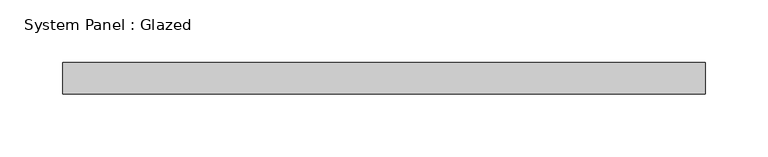
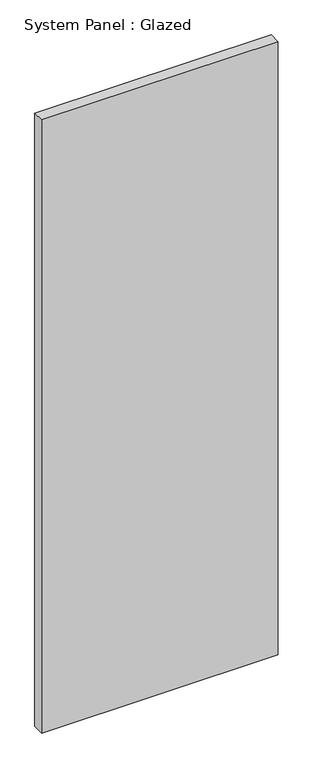
"""IFC4 building model written with IfcOpenShell, lengths in millimetres: plate geometry, System Panel : Glazed."""

from ifc_helpers import new_model, si_unit, origin, origin_with_axes, place, context, project, spatial, polyline, outline, extrude, source, transform, mapped, element, save


def system_panel_glazed_b96b1f03(model_context):
    return source(origin(), model_context, "Body", "SweptSolid", [
        extrude(outline(polyline([(257.175, 19.05), (-257.175, 19.05), (-257.175, 44.45), (257.175, 44.45), (257.175, 19.05)])), origin_with_axes(), (0.0, 0.0, 1.0), 1409.2264761),
    ])


if __name__ == "__main__":
    model = new_model("IFC4")
    model_context = context("Model", 3, world=origin())
    ifc_project = project(units=[si_unit("LENGTHUNIT", "METRE", prefix="MILLI")], contexts=[model_context])
    site = spatial("IfcSite", under=ifc_project)
    building = spatial("IfcBuilding", under=site)
    placement = place(None, origin())
    system_panel_glazed_shape = system_panel_glazed_b96b1f03(model_context)
    element("IfcPlate", 1, ObjectType="System Panel : Glazed", at=placement, inside=building, context=model_context, shape_type="MappedRepresentation", body=[
        mapped(system_panel_glazed_shape, transform((0.0, 0.0, 0.0), x_axis=(1.0, 0.0, 0.0), y_axis=(0.0, 1.0, 0.0), z_axis=(0.0, 0.0, 1.0))),
    ])
    save(model, "model.ifc")

# Revit data of these elements
# Type "System Panel : Glazed"
#   Construction Type Id = "GSP4R"
#   Analytic Construction = "1/8 in Pilkington single glazing"
#   Visual Light Transmittance = 0.9
#   Solar Heat Gain Coefficient = 0.86
#   Heat Transfer Coefficient (U) = 1.18115 BTU/(h·ft²·°F)
#   Define Thermal Properties by = 1
# Element 1 (IfcPlate, "System Panel : Glazed")
#   Materials on its faces: "Glass"
# Materials
#   "Glass": class "Glass", colour RGB 0 128 192, transparency 0.75, Description = "Soda Lime Glass", Cost = 0
